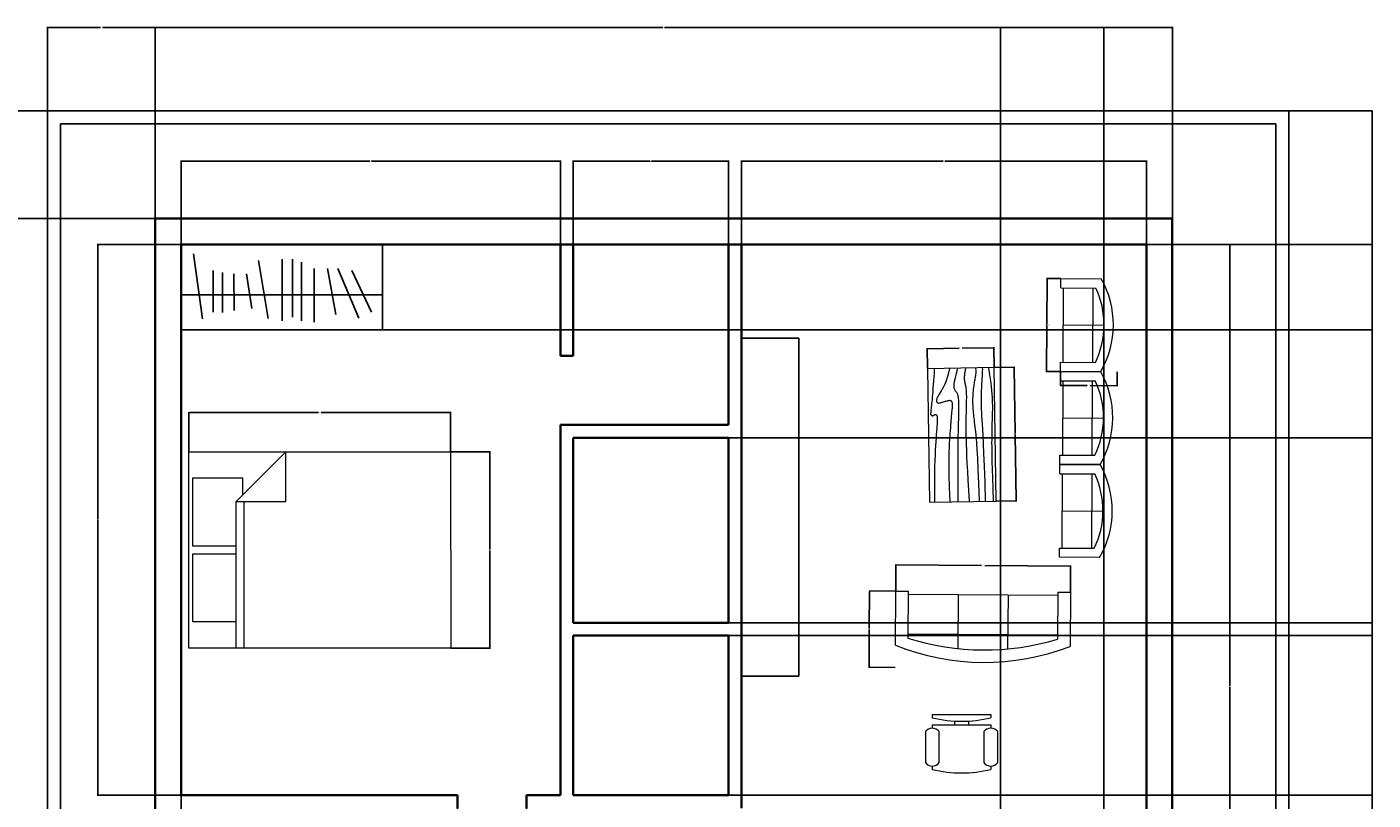
# Model space of a CAD drawing. Units: inches. Extents: x -1085 to 1941, y 1514 to 2348.
# Tile 4 of 9: x -836 to -367, y 2003 to 2272. Entities that reach past the tile are written whole.
import ezdxf

# ---------------------------------------------------------------- set-up
doc = ezdxf.new("R2010")
doc.units = ezdxf.units.IN
for name, color, linetype, lineweight in [('A-ANNO-DIMS', 2, 'Continuous', 18), ('A-FLOR-CASE', 2, 'Continuous', 25), ('A-WALL', 7, 'Continuous', 35), ('C-PROP', 8, 'Continuous', 25), ('FOUNITR-URE', 2, 'Continuous', 18)]:
    doc.layers.add(name, color=color, linetype=linetype, lineweight=lineweight)
doc.styles.get("Standard").update_dxf_attribs({"font": 'arial.ttf'})
doc.dimstyles.get("Standard").update_dxf_attribs({"dimtxt": 0.18, "dimasz": 0.18, "dimexe": 0.18, "dimexo": 0.0625, "dimgap": 0.09, "dimtad": 0, "dimtih": 1, "dimtoh": 1, "dimdec": 4, "dimzin": 0, "dimdsep": 46, "dimtxsty": 'Standard', "dimcen": 0.09, "dimadec": 0, "dimazin": 0, "dimtfac": 1, "dimtdec": 4, "dimtofl": 0, "dimtmove": 0, "dimatfit": 3, "dimfxl": 1, "dimtolj": 1, "dimtzin": 0, "dimarcsym": 0})

# ---------------------------------------------------------------- blocks, each defined once
blk = doc.blocks.new('Bed - Queen')
for p, q in [((0, -80.00003), (0, 0)), ((0, 0), (59.99999, 0)), ((59.99999, 0), (59.99999, -80.00003)), ((7.99999, -1.2), (28.79998, -1.2)), ((7.99999, -14.4), (7.99999, -1.2)), ((28.79998, -1.2), (28.79998, -14.4)), ((31.19999, -1.2), (51.99999, -1.2)), ((31.19999, -14.4), (31.19999, -1.2)), ((51.99999, -1.2), (51.99999, -16.4)), ((0, -14.4), (44.8, -14.4)), ((59.99999, -29.6), (44.8, -14.4)), ((44.8, -14.4), (44.8, -29.6)), ((51.99999, -16.4), (46.79936, -16.4)), ((44.8, -16.8), (0, -16.8)), ((44.8, -29.6), (59.99999, -29.6)), ((59.99999, -80.00003), (0, -80.00003))]:
    blk.add_line(p, q)
blk = doc.blocks.new('Chair - Desk')
for p, q in [((-8.5, 0), (-8.5, -1)), ((-8.5, 0), (8.5, 0)), ((8.5, 0), (8.5, -1)), ((-8.5, -3), (-8.5, -4)), ((-8.5, -3), (8.5, -3)), ((-2, -3), (-2, -1.9355)), ((2, -1.9576), (2, -3)), ((8.5, -3), (8.5, -4)), ((-10.5, -5), (-10.5, -14)), ((-6.5, -14), (-6.5, -5)), ((6.5, -5), (6.5, -14)), ((10.5, -14), (10.5, -5)), ((-8.5, -15), (-8.5, -16)), ((8.5, -15), (8.5, -16))]:
    blk.add_line(p, q)
for centre, radius, start, end in [((0, 34.625), 36.625, 256.5803, 283.4197), ((-8.5, -6.5), 2.5, 36.8699, 143.1301), ((8.5, -6.5), 2.5, 36.8699, 143.1301), ((-8.5, -12.5), 2.5, 216.8699, 323.1301), ((8.5, -12.5), 2.5, 216.8699, 323.1301), ((0, 19.625), 36.625, 256.5803, 283.4197)]:
    blk.add_arc(centre, radius, start, end)
blk = doc.blocks.new('Sofa - Roundback Loveseat 5 ft.')
for p, q in [((0, -32.44198), (0, -5.99998)), ((-24, -33.99998), (-24, -11.46958)), ((-23.9998, -13.38178), (23.99986, -13.38178)), ((24.00004, -33.99998), (24.00004, -11.46958)), ((-24, -32.44198), (24.00004, -32.44198))]:
    blk.add_line(p, q)
for points in [[(-24, -33.99998), (-30, -33.99998), (-30, -7.99998)], [(30.00004, -7.99998), (30.00004, -33.99998), (24.00004, -33.99998)]]:
    blk.add_lwpolyline(points)
for centre, radius, start, end in [((0, -60.24998), 60.24998, 60.13715, 119.8628), ((0, -61.38438), 55.38444, 64.32083, 115.6792)]:
    blk.add_arc(centre, radius, start, end)
blk = doc.blocks.new('Sofa - Roundback 7 ft.')
for p, q in [((-36.000027, -34), (-36.000027, -11.4696)), ((-12.00002, -32.4421), (-12.00003, -6.5971)), ((11.99997, -32.4421), (11.99998, -6.5971)), ((35.99998, -34), (35.99998, -11.4696)), ((-35.999844, -13.3819), (35.9998, -13.3819)), ((-36.000027, -32.4421), (35.99998, -32.4421))]:
    blk.add_line(p, q)
for points in [[(-36.000027, -34), (-42.000027, -34), (-42.000027, -8)], [(41.99998, -8), (41.99998, -34), (35.99998, -34)]]:
    blk.add_lwpolyline(points)
for centre, radius, start, end in [((0, -114.25), 114.25, 68.43141, 111.5686), ((-0.00001, -127.1968), 121.1968, 72.72033, 107.2797)]:
    blk.add_arc(centre, radius, start, end)
blk = doc.blocks.new('Table - Rectangular Woodgrain 60 x 30 in.')
for p, q in [((0, 0), (0, -30)), ((60, 0), (0, 0)), ((60, -30), (60, 0)), ((0, -30), (60, -30))]:
    blk.add_line(p, q)
for points in [[(0, -2.4), (4.8155, -2.418), (9.0302, -2.4688), (12.709, -2.5477), (15.9167, -2.65), (18.7181, -2.7711), (21.1781, -2.9063), (23.3616, -3.0508), (25.3333, -3.2), (27.1477, -3.3495), (28.8172, -3.4958), (30.3437, -3.636), (31.7291, -3.7667), (32.9756, -3.8849), (34.0849, -3.9875), (35.059, -4.0714), (35.9, -4.1334), (36.6114, -4.1711), (37.2041, -4.1854), (37.6906, -4.1779), (38.0833, -4.15), (38.3948, -4.1034), (38.6375, -4.0396), (38.8239, -3.9602), (38.9666, -3.8667), (39.0764, -3.7608), (39.1573, -3.6448), (39.2116, -3.521), (39.2416, -3.3917), (39.2498, -3.2593), (39.2385, -3.1261), (39.21, -2.9944), (39.1666, -2.8667), (39.111, -2.7447), (39.0468, -2.6281), (38.978, -2.5163), (38.9083, -2.4083), (38.8418, -2.3035), (38.7823, -2.201), (38.7337, -2.1001), (38.7, -2), (38.6844, -1.9003), (38.6875, -1.8021), (38.7094, -1.707), (38.75, -1.6167), (38.8094, -1.5326), (38.8875, -1.4563), (38.9844, -1.3893), (39.1, -1.3333), (39.2351, -1.2896), (39.3937, -1.2583), (39.5804, -1.2396), (39.8, -1.2333), (40.057, -1.2396), (40.3562, -1.2583), (40.7023, -1.2896), (41.1, -1.3333), (41.5547, -1.3895), (42.0755, -1.4573), (42.6721, -1.5361), (43.3542, -1.625), (44.1316, -1.7233), (45.014, -1.8302), (46.0114, -1.9449), (47.1333, -2.0667), (48.3862, -2.1947), (49.7625, -2.3281), (51.2513, -2.4663), (52.8416, -2.6083), (54.5226, -2.7535), (56.2833, -2.9011), (58.1127, -3.0501), (60, -3.2)], [(0, -9.2), (6.5759, -9.0858), (11.9385, -9.0365), (16.2527, -9.0418), (19.6833, -9.0917), (22.3952, -9.1759), (24.5531, -9.2844), (26.322, -9.4069), (27.8666, -9.5333), (29.3241, -9.6553), (30.7203, -9.7719), (32.0532, -9.8837), (33.3208, -9.9917), (34.5213, -10.0965), (35.6526, -10.199), (36.7128, -10.2999), (37.7, -10.4), (38.6129, -10.4996), (39.4531, -10.5969), (40.223, -10.6895), (40.925, -10.775), (41.5613, -10.8512), (42.1344, -10.9156), (42.6465, -10.966), (43.1, -11), (43.4976, -11.0158), (43.8437, -11.0136), (44.143, -10.9942), (44.4, -10.9583), (44.6195, -10.9069), (44.8062, -10.8406), (44.9648, -10.7603), (45.1, -10.6667), (45.2155, -10.5598), (45.3114, -10.4365), (45.3871, -10.2929), (45.4416, -10.125), (45.4743, -9.929), (45.4844, -9.7011), (45.4709, -9.4371), (45.4333, -9.1333), (45.3716, -8.7883), (45.2896, -8.4104), (45.1919, -8.0107), (45.0833, -7.6), (44.9685, -7.1893), (44.8521, -6.7896), (44.7388, -6.4117), (44.6333, -6.0667), (44.54, -5.7628), (44.4614, -5.4979), (44.4001, -5.2675), (44.3583, -5.0667), (44.3384, -4.8909), (44.3427, -4.7354), (44.3736, -4.5956), (44.4333, -4.4667), (44.5236, -4.3453), (44.6427, -4.2333), (44.7884, -4.1339), (44.9583, -4.05), (45.1501, -3.9849), (45.3614, -3.9417), (45.59, -3.9234), (45.8333, -3.9333), (46.0915, -3.9749), (46.3734, -4.0531), (46.6906, -4.1736), (47.0542, -4.3417), (47.4756, -4.5629), (47.9661, -4.8427), (48.5372, -5.1866), (49.2, -5.6), (49.9676, -6.0844), (50.8594, -6.625), (51.8965, -7.2031), (53.1, -7.8), (54.491, -8.3969), (56.0906, -8.975), (57.9199, -9.5156), (60, -10)], [(0, -12.8), (5.1847, -12.9322), (9.6213, -13.0323), (13.3963, -13.1059), (16.5958, -13.1583), (19.3063, -13.1952), (21.614, -13.2219), (23.6054, -13.2439), (25.3666, -13.2667), (26.9728, -13.2947), (28.4531, -13.3281), (29.8256, -13.3663), (31.1083, -13.4083), (32.3191, -13.4535), (33.476, -13.501), (34.597, -13.5501), (35.7, -13.6), (36.7984, -13.6497), (37.8875, -13.6979), (38.9578, -13.743), (40, -13.7833), (41.0047, -13.8174), (41.9625, -13.8438), (42.864, -13.8607), (43.7, -13.8667), (44.4631, -13.8604), (45.1552, -13.8417), (45.7801, -13.8104), (46.3416, -13.7667), (46.8439, -13.7104), (47.2906, -13.6417), (47.6858, -13.5604), (48.0333, -13.4667), (48.3375, -13.3608), (48.6042, -13.2448), (48.8396, -13.121), (49.05, -12.9917), (49.2417, -12.8593), (49.4208, -12.7261), (49.5937, -12.5944), (49.7667, -12.4667), (49.9452, -12.3451), (50.1323, -12.2313), (50.3303, -12.1268), (50.5416, -12.0333), (50.7686, -11.9524), (51.0135, -11.8854), (51.2788, -11.8341), (51.5666, -11.8), (51.8785, -11.7843), (52.2116, -11.7865), (52.562, -11.8059), (52.926, -11.8417), (53.2998, -11.8931), (53.6795, -11.9594), (54.0614, -12.0397), (54.4416, -12.1333), (54.8223, -12.2401), (55.2293, -12.3625), (55.6942, -12.5037), (56.2489, -12.6667), (56.9251, -12.8547), (57.7545, -13.0708), (58.7689, -13.3182), (60, -13.6)], [(0, -18), (5.124, -17.7273), (9.6609, -17.5057), (13.6705, -17.3303), (17.2125, -17.1958), (20.3467, -17.0973), (23.1328, -17.0297), (25.6307, -16.9878), (27.9, -16.9667), (29.9928, -16.9617), (31.9302, -16.9703), (33.7254, -16.9907), (35.3917, -17.0208), (36.9423, -17.0588), (38.3906, -17.1026), (39.7499, -17.1503), (41.0333, -17.2), (42.2519, -17.2496), (43.4073, -17.2969), (44.4986, -17.3395), (45.525, -17.375), (46.4858, -17.4012), (47.3802, -17.4156), (48.2074, -17.416), (48.9667, -17.4), (49.6583, -17.3662), (50.2872, -17.3167), (50.8595, -17.2547), (51.3812, -17.1833), (51.8584, -17.1057), (52.2971, -17.025), (52.7034, -16.9443), (53.0833, -16.8667), (53.443, -16.7951), (53.789, -16.7313), (54.128, -16.6768), (54.4666, -16.6334), (54.8115, -16.6024), (55.1693, -16.5854), (55.5465, -16.5841), (55.95, -16.6), (56.3828, -16.6337), (56.8346, -16.6823), (57.2915, -16.7418), (57.7396, -16.8084), (58.165, -16.878), (58.5539, -16.9469), (58.8924, -17.0111), (59.1666, -17.0667), (59.3679, -17.1107), (59.5078, -17.1438), (59.6032, -17.1675), (59.6708, -17.1833), (59.7275, -17.193), (59.7901, -17.1979), (59.8753, -17.1998), (60, -17.2)], [(0, -22.4), (8.0098, -22.2501), (14.4094, -22.1011), (19.4168, -21.9535), (23.25, -21.8083), (26.1269, -21.6663), (28.2656, -21.5281), (29.884, -21.3947), (31.2, -21.2667), (32.3967, -21.1448), (33.5172, -21.0292), (34.5697, -20.9198), (35.5625, -20.8167), (36.5037, -20.7198), (37.4015, -20.6292), (38.2642, -20.5448), (39.1, -20.4667), (39.9164, -20.3951), (40.7187, -20.3313), (41.5117, -20.2768), (42.3, -20.2333), (43.0883, -20.2024), (43.8812, -20.1854), (44.6836, -20.1841), (45.5, -20.2), (46.3328, -20.234), (47.1747, -20.2844), (48.0163, -20.3488), (48.8479, -20.425), (49.66, -20.5106), (50.4429, -20.6031), (51.1872, -20.7004), (51.8833, -20.8), (52.5246, -20.8999), (53.1166, -20.9995), (53.6681, -21.0983), (54.1875, -21.1958), (54.6834, -21.2919), (55.1646, -21.3859), (55.6394, -21.4777), (56.1167, -21.5667), (56.6028, -21.6515), (57.0961, -21.7266), (57.5929, -21.7852), (58.0896, -21.8208), (58.5823, -21.8268), (59.0674, -21.7964), (59.5412, -21.723), (60, -21.6)], [(0, -25.2), (8.6355, -25.0504), (15.7026, -24.9031), (21.4049, -24.7606), (25.9458, -24.625), (29.529, -24.4988), (32.3578, -24.3844), (34.6359, -24.284), (36.5667, -24.2), (38.3213, -24.1341), (39.9417, -24.0854), (41.437, -24.0523), (42.8167, -24.0333), (44.0901, -24.0268), (45.2667, -24.0313), (46.3557, -24.0451), (47.3667, -24.0667), (48.309, -24.0947), (49.1928, -24.1287), (50.0284, -24.168), (50.826, -24.2125), (51.5959, -24.2617), (52.3483, -24.3151), (53.0935, -24.3725), (53.8417, -24.4334), (54.6009, -24.497), (55.3699, -24.561), (56.1454, -24.6226), (56.9239, -24.6792), (57.7021, -24.7279), (58.4764, -24.7662), (59.2435, -24.7911), (60, -24.8)], [(0, -28.8), (5.6867, -28.6681), (10.45, -28.5698), (14.407, -28.5012), (17.675, -28.4584), (20.3711, -28.4374), (22.6125, -28.4344), (24.5164, -28.4455), (26.2, -28.4667), (27.762, -28.4947), (29.2276, -28.5281), (30.6033, -28.5663), (31.8958, -28.6084), (33.1118, -28.6535), (34.2578, -28.7011), (35.3405, -28.7501), (36.3666, -28.8), (37.3443, -28.8497), (38.288, -28.8974), (39.2137, -28.9412), (40.1375, -28.9792), (41.0753, -29.0093), (42.0432, -29.0297), (43.0572, -29.0384), (44.1333, -29.0333), (45.2936, -29.0114), (46.5843, -28.9641), (48.0579, -28.8816), (49.7666, -28.7542), (51.7629, -28.5721), (54.0989, -28.3255), (56.8272, -28.0048), (60, -27.6)]]:
    blk.add_lwpolyline(points)
blk = doc.blocks.new('*D36')
at = {"layer": 'A-ANNO-DIMS', "color": 0, "lineweight": -2, "transparency": 16777216}
for p, q in [((-779.4, 2124.23), (-779.4, 2138.01)), ((-779.22, 2137.83), (-734.35, 2137.84)), ((-688.49, 2137.86), (-733.36, 2137.84)), ((-688.3, 2124.25), (-688.31, 2138.04))]:
    blk.add_line(p, q, dxfattribs=at)
at = {"layer": 'A-ANNO-DIMS', "color": 0, "transparency": 16777216}
for points in [[(-779.22, 2137.86), (-779.22, 2137.8), (-779.4, 2137.83)], [(-688.49, 2137.89), (-688.49, 2137.83), (-688.31, 2137.86)]]:
    blk.add_solid(points, dxfattribs=at)
at = {"layer": 'Defpoints', "color": 0, "transparency": 16777216}
for p in [(-779.4, 2137.83), (-779.4, 2124.17), (-688.3, 2124.19)]:
    blk.add_point(p, dxfattribs=at)
at = {"layer": 'A-ANNO-DIMS', "color": 0, "transparency": 16777216, "insert": (-733.86, 2137.84), "char_height": 0.18, "attachment_point": 5}
blk.add_mtext('\\A1;BED 91', dxfattribs=at)
blk = doc.blocks.new('*D37')
at = {"layer": 'A-ANNO-DIMS', "color": 0, "lineweight": -2, "transparency": 16777216}
for p, q in [((-688.24, 2124.19), (-674.46, 2124.2)), ((-674.64, 2124.02), (-674.63, 2090.22)), ((-674.62, 2056.05), (-674.63, 2089.85)), ((-688.22, 2055.87), (-674.44, 2055.87))]:
    blk.add_line(p, q, dxfattribs=at)
at = {"layer": 'A-ANNO-DIMS', "color": 0, "transparency": 16777216}
for points in [[(-674.61, 2124.02), (-674.67, 2124.02), (-674.64, 2124.2)], [(-674.59, 2056.05), (-674.65, 2056.05), (-674.62, 2055.87)]]:
    blk.add_solid(points, dxfattribs=at)
at = {"layer": 'Defpoints', "color": 0, "transparency": 16777216}
for p in [(-688.3, 2124.19), (-674.64, 2124.2), (-688.28, 2055.87)]:
    blk.add_point(p, dxfattribs=at)
at = {"layer": 'A-ANNO-DIMS', "color": 0, "transparency": 16777216, "insert": (-674.63, 2090.03), "char_height": 0.18, "attachment_point": 5}
blk.add_mtext('\\A1;68', dxfattribs=at)
blk = doc.blocks.new('*D38')
at = {"layer": 'A-ANNO-DIMS', "color": 0, "lineweight": -2, "transparency": 16777216}
for p, q in [((-475.93, 2184.49), (-480.9, 2184.52)), ((-480.72, 2184.34), (-480.81, 2168.53)), ((-480.9, 2152.35), (-480.81, 2168.16)), ((-476.12, 2152.14), (-481.09, 2152.17))]:
    blk.add_line(p, q, dxfattribs=at)
at = {"layer": 'A-ANNO-DIMS', "color": 0, "transparency": 16777216}
for points in [[(-480.75, 2184.34), (-480.69, 2184.34), (-480.72, 2184.52)], [(-480.93, 2152.35), (-480.87, 2152.35), (-480.91, 2152.17)]]:
    blk.add_solid(points, dxfattribs=at)
at = {"layer": 'Defpoints', "color": 0, "transparency": 16777216}
for p in [(-475.87, 2184.49), (-480.91, 2152.17), (-476.05, 2152.14)]:
    blk.add_point(p, dxfattribs=at)
at = {"layer": 'A-ANNO-DIMS', "color": 0, "transparency": 16777216, "insert": (-480.81, 2168.34), "char_height": 0.18, "attachment_point": 5}
blk.add_mtext('\\A1;LOVESEAT 32 TYP.', dxfattribs=at)
blk = doc.blocks.new('*D39')
at = {"layer": 'A-ANNO-DIMS', "color": 0, "lineweight": -2, "transparency": 16777216}
for p, q in [((-476.05, 2152.08), (-476.08, 2147.11)), ((-456.29, 2151.97), (-456.31, 2147)), ((-475.9, 2147.29), (-466.73, 2147.24)), ((-456.49, 2147.18), (-465.67, 2147.23))]:
    blk.add_line(p, q, dxfattribs=at)
at = {"layer": 'A-ANNO-DIMS', "color": 0, "transparency": 16777216}
for points in [[(-475.9, 2147.32), (-475.9, 2147.26), (-476.08, 2147.29)], [(-456.49, 2147.21), (-456.49, 2147.15), (-456.31, 2147.18)]]:
    blk.add_solid(points, dxfattribs=at)
at = {"layer": 'Defpoints', "color": 0, "transparency": 16777216}
for p in [(-476.05, 2152.14), (-456.29, 2152.03), (-456.31, 2147.18)]:
    blk.add_point(p, dxfattribs=at)
at = {"layer": 'A-ANNO-DIMS', "color": 0, "transparency": 16777216, "insert": (-466.2, 2147.23), "char_height": 0.18, "attachment_point": 5}
blk.add_mtext('\\A1;20 TYP.', dxfattribs=at)
blk = doc.blocks.new('*D44')
at = {"layer": 'A-ANNO-DIMS', "color": 0, "lineweight": -2, "transparency": 16777216}
for p, q in [((-533.37, 2075.73), (-533.31, 2084.97)), ((-533.13, 2084.79), (-503.49, 2084.59)), ((-472.7, 2084.39), (-502.34, 2084.59)), ((-472.58, 2075.33), (-472.52, 2084.57))]:
    blk.add_line(p, q, dxfattribs=at)
at = {"layer": 'A-ANNO-DIMS', "color": 0, "transparency": 16777216}
for points in [[(-533.13, 2084.82), (-533.13, 2084.76), (-533.31, 2084.79)], [(-472.7, 2084.42), (-472.7, 2084.36), (-472.52, 2084.39)]]:
    blk.add_solid(points, dxfattribs=at)
at = {"layer": 'Defpoints', "color": 0, "transparency": 16777216}
for p in [(-533.31, 2084.79), (-533.37, 2075.67), (-472.58, 2075.27)]:
    blk.add_point(p, dxfattribs=at)
at = {"layer": 'A-ANNO-DIMS', "color": 0, "transparency": 16777216, "insert": (-502.92, 2084.59), "char_height": 0.18, "attachment_point": 5}
blk.add_mtext('\\A1;SOFA 61', dxfattribs=at)
blk = doc.blocks.new('*D45')
at = {"layer": 'A-ANNO-DIMS', "color": 0, "lineweight": -2, "transparency": 16777216}
for p, q in [((-533.44, 2075.67), (-542.67, 2075.73)), ((-542.5, 2075.55), (-542.58, 2062.64)), ((-542.67, 2049.37), (-542.58, 2062.28)), ((-533.61, 2049.13), (-542.85, 2049.19))]:
    blk.add_line(p, q, dxfattribs=at)
at = {"layer": 'A-ANNO-DIMS', "color": 0, "transparency": 16777216}
for points in [[(-542.53, 2075.55), (-542.47, 2075.55), (-542.49, 2075.73)], [(-542.7, 2049.37), (-542.64, 2049.37), (-542.67, 2049.19)]]:
    blk.add_solid(points, dxfattribs=at)
at = {"layer": 'Defpoints', "color": 0, "transparency": 16777216}
for p in [(-533.37, 2075.67), (-542.67, 2049.19), (-533.55, 2049.13)]:
    blk.add_point(p, dxfattribs=at)
at = {"layer": 'A-ANNO-DIMS', "color": 0, "transparency": 16777216, "insert": (-542.58, 2062.46), "char_height": 0.18, "attachment_point": 5}
blk.add_mtext('\\A1;27', dxfattribs=at)
blk = doc.blocks.new('*D50')
at = {"layer": 'A-ANNO-DIMS', "color": 0, "lineweight": -2, "transparency": 16777216}
for p, q in [((-499.03, 2153.46), (-491.95, 2153.58)), ((-492.13, 2153.39), (-491.77, 2130.54)), ((-491.4, 2107.32), (-491.76, 2130.18)), ((-498.3, 2107.03), (-491.22, 2107.15))]:
    blk.add_line(p, q, dxfattribs=at)
at = {"layer": 'A-ANNO-DIMS', "color": 0, "transparency": 16777216}
for points in [[(-492.1, 2153.39), (-492.16, 2153.39), (-492.13, 2153.57)], [(-491.37, 2107.32), (-491.43, 2107.32), (-491.4, 2107.14)]]:
    blk.add_solid(points, dxfattribs=at)
at = {"layer": 'Defpoints', "color": 0, "transparency": 16777216}
for p in [(-499.1, 2153.46), (-492.13, 2153.57), (-498.36, 2107.03)]:
    blk.add_point(p, dxfattribs=at)
at = {"layer": 'A-ANNO-DIMS', "color": 0, "transparency": 16777216, "insert": (-491.77, 2130.36), "char_height": 0.18, "attachment_point": 5}
blk.add_mtext('\\A1;TABLE 46 TYP.', dxfattribs=at)
blk = doc.blocks.new('*D51')
at = {"layer": 'A-ANNO-DIMS', "color": 0, "lineweight": -2, "transparency": 16777216}
for p, q in [((-522.31, 2153.16), (-522.42, 2160.24)), ((-522.24, 2160.06), (-511.34, 2160.24)), ((-499.39, 2160.42), (-510.28, 2160.25)), ((-499.1, 2153.53), (-499.21, 2160.61))]:
    blk.add_line(p, q, dxfattribs=at)
at = {"layer": 'A-ANNO-DIMS', "color": 0, "transparency": 16777216}
for points in [[(-522.24, 2160.09), (-522.24, 2160.03), (-522.42, 2160.06)], [(-499.39, 2160.45), (-499.39, 2160.39), (-499.21, 2160.43)]]:
    blk.add_solid(points, dxfattribs=at)
at = {"layer": 'Defpoints', "color": 0, "transparency": 16777216}
for p in [(-522.42, 2160.06), (-522.31, 2153.1), (-499.1, 2153.46)]:
    blk.add_point(p, dxfattribs=at)
at = {"layer": 'A-ANNO-DIMS', "color": 0, "transparency": 16777216, "insert": (-510.81, 2160.24), "char_height": 0.18, "attachment_point": 5}
blk.add_mtext('\\A1;23 TYP.', dxfattribs=at)
blk = doc.blocks.new('*D95')
at = {"layer": 'A-ANNO-DIMS', "color": 0, "lineweight": -2, "transparency": 16777216}
for p, q in [((-396.54, 2242.88), (-367.42, 2242.88)), ((-367.6, 2242.7), (-367.6, 1955.07)), ((-367.6, 1667.06), (-367.6, 1954.7)), ((-396.54, 1666.88), (-367.42, 1666.88))]:
    blk.add_line(p, q, dxfattribs=at)
at = {"layer": 'A-ANNO-DIMS', "color": 0, "transparency": 16777216}
for points in [[(-367.63, 2242.7), (-367.57, 2242.7), (-367.6, 2242.88)], [(-367.63, 1667.06), (-367.57, 1667.06), (-367.6, 1666.88)]]:
    blk.add_solid(points, dxfattribs=at)
at = {"layer": 'Defpoints', "color": 0, "transparency": 16777216}
for p in [(-396.6, 2242.88), (-367.6, 2242.88), (-396.6, 1666.88)]:
    blk.add_point(p, dxfattribs=at)
at = {"layer": 'A-ANNO-DIMS', "color": 0, "transparency": 16777216, "insert": (-367.6, 1954.88), "char_height": 0.18, "attachment_point": 5}
blk.add_mtext('\\A1;576', dxfattribs=at)
blk = doc.blocks.new('*D96')
at = {"layer": 'A-ANNO-DIMS', "color": 0, "lineweight": -2, "transparency": 16777216}
for p, q in [((-791.1, 2205.45), (-791.1, 2272.06)), ((-790.92, 2271.88), (-614.39, 2271.88)), ((-437.28, 2271.88), (-613.81, 2271.88)), ((-437.1, 2205.45), (-437.1, 2272.06))]:
    blk.add_line(p, q, dxfattribs=at)
at = {"layer": 'A-ANNO-DIMS', "color": 0, "transparency": 16777216}
for points in [[(-790.92, 2271.91), (-790.92, 2271.85), (-791.1, 2271.88)], [(-437.28, 2271.91), (-437.28, 2271.85), (-437.1, 2271.88)]]:
    blk.add_solid(points, dxfattribs=at)
at = {"layer": 'Defpoints', "color": 0, "transparency": 16777216}
for p in [(-437.1, 2271.88), (-791.1, 2205.38), (-437.1, 2205.38)]:
    blk.add_point(p, dxfattribs=at)
at = {"layer": 'A-ANNO-DIMS', "color": 0, "transparency": 16777216, "insert": (-614.1, 2271.88), "char_height": 0.18, "attachment_point": 5}
blk.add_mtext('\\A1;354', dxfattribs=at)
blk = doc.blocks.new('*D97')
at = {"layer": 'A-ANNO-DIMS', "color": 0, "lineweight": -2, "transparency": 16777216}
for p, q in [((-791.17, 2205.38), (-857.78, 2205.38)), ((-857.6, 2205.2), (-857.6, 1965.57)), ((-857.6, 1725.56), (-857.6, 1965.2)), ((-791.17, 1725.38), (-857.78, 1725.38))]:
    blk.add_line(p, q, dxfattribs=at)
at = {"layer": 'A-ANNO-DIMS', "color": 0, "transparency": 16777216}
for points in [[(-857.63, 2205.2), (-857.57, 2205.2), (-857.6, 2205.38)], [(-857.63, 1725.56), (-857.57, 1725.56), (-857.6, 1725.38)]]:
    blk.add_solid(points, dxfattribs=at)
at = {"layer": 'Defpoints', "color": 0, "transparency": 16777216}
for p in [(-791.1, 2205.38), (-857.6, 1725.38), (-791.1, 1725.38)]:
    blk.add_point(p, dxfattribs=at)
at = {"layer": 'A-ANNO-DIMS', "color": 0, "transparency": 16777216, "insert": (-857.6, 1965.38), "char_height": 0.18, "attachment_point": 5}
blk.add_mtext('\\A1;480', dxfattribs=at)
blk = doc.blocks.new('*D98')
at = {"layer": 'A-ANNO-DIMS', "color": 0, "lineweight": -2, "transparency": 16777216}
for p, q in [((-828.6, 2242.95), (-828.6, 2272.06)), ((-828.42, 2271.88), (-810.18, 2271.88)), ((-791.28, 2271.88), (-809.53, 2271.88)), ((-791.1, 2205.45), (-791.1, 2272.06))]:
    blk.add_line(p, q, dxfattribs=at)
at = {"layer": 'A-ANNO-DIMS', "color": 0, "transparency": 16777216}
for points in [[(-828.42, 2271.91), (-828.42, 2271.85), (-828.6, 2271.88)], [(-791.28, 2271.91), (-791.28, 2271.85), (-791.1, 2271.88)]]:
    blk.add_solid(points, dxfattribs=at)
at = {"layer": 'Defpoints', "color": 0, "transparency": 16777216}
for p in [(-791.1, 2271.88), (-828.6, 2242.88), (-791.1, 2205.38)]:
    blk.add_point(p, dxfattribs=at)
at = {"layer": 'A-ANNO-DIMS', "color": 0, "transparency": 16777216, "insert": (-809.85, 2271.88), "char_height": 0.18, "attachment_point": 5}
blk.add_mtext('\\A1;37.5', dxfattribs=at)
blk = doc.blocks.new('*D99')
at = {"layer": 'A-ANNO-DIMS', "color": 0, "lineweight": -2, "transparency": 16777216}
for p, q in [((-828.67, 2242.88), (-857.78, 2242.88)), ((-857.6, 2242.7), (-857.6, 2224.32)), ((-857.6, 2205.56), (-857.6, 2223.95)), ((-791.17, 2205.38), (-857.78, 2205.38))]:
    blk.add_line(p, q, dxfattribs=at)
at = {"layer": 'A-ANNO-DIMS', "color": 0, "transparency": 16777216}
for points in [[(-857.63, 2242.7), (-857.57, 2242.7), (-857.6, 2242.88)], [(-857.63, 2205.56), (-857.57, 2205.56), (-857.6, 2205.38)]]:
    blk.add_solid(points, dxfattribs=at)
at = {"layer": 'Defpoints', "color": 0, "transparency": 16777216}
for p in [(-828.6, 2242.88), (-857.6, 2205.38), (-791.1, 2205.38)]:
    blk.add_point(p, dxfattribs=at)
at = {"layer": 'A-ANNO-DIMS', "color": 0, "transparency": 16777216, "insert": (-857.6, 2224.13), "char_height": 0.18, "attachment_point": 5}
blk.add_mtext('\\A1;37.5', dxfattribs=at)
blk = doc.blocks.new('*D100')
at = {"layer": 'A-ANNO-DIMS', "color": 0, "lineweight": -2, "transparency": 16777216}
for p, q in [((-782.1, 2196.45), (-782.1, 2225.56)), ((-781.92, 2225.38), (-716.38, 2225.38)), ((-650.28, 2225.38), (-715.82, 2225.38)), ((-650.1, 2196.45), (-650.1, 2225.56))]:
    blk.add_line(p, q, dxfattribs=at)
at = {"layer": 'A-ANNO-DIMS', "color": 0, "transparency": 16777216}
for points in [[(-781.92, 2225.41), (-781.92, 2225.35), (-782.1, 2225.38)], [(-650.28, 2225.41), (-650.28, 2225.35), (-650.1, 2225.38)]]:
    blk.add_solid(points, dxfattribs=at)
at = {"layer": 'Defpoints', "color": 0, "transparency": 16777216}
for p in [(-650.1, 2225.38), (-782.1, 2196.38), (-650.1, 2196.38)]:
    blk.add_point(p, dxfattribs=at)
at = {"layer": 'A-ANNO-DIMS', "color": 0, "transparency": 16777216, "insert": (-716.1, 2225.38), "char_height": 0.18, "attachment_point": 5}
blk.add_mtext('\\A1;132', dxfattribs=at)
blk = doc.blocks.new('*D101')
at = {"layer": 'A-ANNO-DIMS', "color": 0, "lineweight": -2, "transparency": 16777216}
for p, q in [((-782.17, 2196.38), (-811.28, 2196.38)), ((-811.1, 2196.2), (-811.1, 2100.71)), ((-811.1, 2004.86), (-811.1, 2100.35)), ((-782.17, 2004.68), (-811.28, 2004.68))]:
    blk.add_line(p, q, dxfattribs=at)
at = {"layer": 'A-ANNO-DIMS', "color": 0, "transparency": 16777216}
for points in [[(-811.13, 2196.2), (-811.07, 2196.2), (-811.1, 2196.38)], [(-811.13, 2004.86), (-811.07, 2004.86), (-811.1, 2004.68)]]:
    blk.add_solid(points, dxfattribs=at)
at = {"layer": 'Defpoints', "color": 0, "transparency": 16777216}
for p in [(-811.1, 2196.38), (-782.1, 2196.38), (-782.1, 2004.68)]:
    blk.add_point(p, dxfattribs=at)
at = {"layer": 'A-ANNO-DIMS', "color": 0, "transparency": 16777216, "insert": (-811.1, 2100.53), "char_height": 0.18, "attachment_point": 5}
blk.add_mtext('\\A1;191.7', dxfattribs=at)
blk = doc.blocks.new('*D102')
at = {"layer": 'A-ANNO-DIMS', "color": 0, "lineweight": -2, "transparency": 16777216}
for p, q in [((-645.6, 2196.45), (-645.6, 2225.56)), ((-645.42, 2225.38), (-618.82, 2225.38)), ((-591.78, 2225.38), (-618.38, 2225.38)), ((-591.6, 2196.45), (-591.6, 2225.56))]:
    blk.add_line(p, q, dxfattribs=at)
at = {"layer": 'A-ANNO-DIMS', "color": 0, "transparency": 16777216}
for points in [[(-645.42, 2225.41), (-645.42, 2225.35), (-645.6, 2225.38)], [(-591.78, 2225.41), (-591.78, 2225.35), (-591.6, 2225.38)]]:
    blk.add_solid(points, dxfattribs=at)
at = {"layer": 'Defpoints', "color": 0, "transparency": 16777216}
for p in [(-591.6, 2225.38), (-645.6, 2196.38), (-591.6, 2196.38)]:
    blk.add_point(p, dxfattribs=at)
at = {"layer": 'A-ANNO-DIMS', "color": 0, "transparency": 16777216, "insert": (-618.6, 2225.38), "char_height": 0.18, "attachment_point": 5}
blk.add_mtext('\\A1;54', dxfattribs=at)
blk = doc.blocks.new('*D103')
at = {"layer": 'A-ANNO-DIMS', "color": 0, "lineweight": -2, "transparency": 16777216}
for p, q in [((-645.54, 2060.18), (-367.42, 2060.18)), ((-367.6, 2060), (-367.6, 2032.61)), ((-367.6, 2004.86), (-367.6, 2032.25)), ((-645.54, 2004.68), (-367.42, 2004.68))]:
    blk.add_line(p, q, dxfattribs=at)
at = {"layer": 'A-ANNO-DIMS', "color": 0, "transparency": 16777216}
for points in [[(-367.63, 2060), (-367.57, 2060), (-367.6, 2060.18)], [(-367.63, 2004.86), (-367.57, 2004.86), (-367.6, 2004.68)]]:
    blk.add_solid(points, dxfattribs=at)
at = {"layer": 'Defpoints', "color": 0, "transparency": 16777216}
for p in [(-645.6, 2060.18), (-367.6, 2060.18), (-645.6, 2004.68)]:
    blk.add_point(p, dxfattribs=at)
at = {"layer": 'A-ANNO-DIMS', "color": 0, "transparency": 16777216, "insert": (-367.6, 2032.43), "char_height": 0.18, "attachment_point": 5}
blk.add_mtext('\\A1;55.5', dxfattribs=at)
blk = doc.blocks.new('*D104')
at = {"layer": 'A-ANNO-DIMS', "color": 0, "lineweight": -2, "transparency": 16777216}
for p, q in [((-645.54, 2129.05), (-367.42, 2129.05)), ((-367.6, 2128.87), (-367.6, 2097.05)), ((-367.6, 2064.86), (-367.6, 2096.68)), ((-645.54, 2064.68), (-367.42, 2064.68))]:
    blk.add_line(p, q, dxfattribs=at)
at = {"layer": 'A-ANNO-DIMS', "color": 0, "transparency": 16777216}
for points in [[(-367.63, 2128.87), (-367.57, 2128.87), (-367.6, 2129.05)], [(-367.63, 2064.86), (-367.57, 2064.86), (-367.6, 2064.68)]]:
    blk.add_solid(points, dxfattribs=at)
at = {"layer": 'Defpoints', "color": 0, "transparency": 16777216}
for p in [(-645.6, 2129.05), (-367.6, 2129.05), (-645.6, 2064.68)]:
    blk.add_point(p, dxfattribs=at)
at = {"layer": 'A-ANNO-DIMS', "color": 0, "transparency": 16777216, "insert": (-367.6, 2096.87), "char_height": 0.18, "attachment_point": 5}
blk.add_mtext('\\A1;64.38', dxfattribs=at)
blk = doc.blocks.new('*D105')
at = {"layer": 'A-ANNO-DIMS', "color": 0, "lineweight": -2, "transparency": 16777216}
for p, q in [((-782.04, 2196.38), (-367.42, 2196.38)), ((-367.6, 2196.2), (-367.6, 2181.71)), ((-367.6, 2166.86), (-367.6, 2181.35)), ((-782.04, 2166.68), (-367.42, 2166.68))]:
    blk.add_line(p, q, dxfattribs=at)
at = {"layer": 'A-ANNO-DIMS', "color": 0, "transparency": 16777216}
for points in [[(-367.63, 2196.2), (-367.57, 2196.2), (-367.6, 2196.38)], [(-367.63, 2166.86), (-367.57, 2166.86), (-367.6, 2166.68)]]:
    blk.add_solid(points, dxfattribs=at)
at = {"layer": 'Defpoints', "color": 0, "transparency": 16777216}
for p in [(-782.1, 2196.38), (-782.1, 2166.68), (-367.6, 2166.68)]:
    blk.add_point(p, dxfattribs=at)
at = {"layer": 'A-ANNO-DIMS', "color": 0, "transparency": 16777216, "insert": (-367.6, 2181.53), "char_height": 0.18, "attachment_point": 5}
blk.add_mtext('\\A1;29.706', dxfattribs=at)
blk = doc.blocks.new('*D106')
at = {"layer": 'A-ANNO-DIMS', "color": 0, "lineweight": -2, "transparency": 16777216}
for p, q in [((-685.88, 2004.62), (-685.88, 1637.7)), ((-661.88, 2004.62), (-661.88, 1637.7)), ((-685.7, 1637.88), (-674.1, 1637.88)), ((-662.06, 1637.88), (-673.66, 1637.88))]:
    blk.add_line(p, q, dxfattribs=at)
at = {"layer": 'A-ANNO-DIMS', "color": 0, "transparency": 16777216}
for points in [[(-685.7, 1637.91), (-685.7, 1637.85), (-685.88, 1637.88)], [(-662.06, 1637.91), (-662.06, 1637.85), (-661.88, 1637.88)]]:
    blk.add_solid(points, dxfattribs=at)
at = {"layer": 'Defpoints', "color": 0, "transparency": 16777216}
for p in [(-685.88, 2004.68), (-661.88, 2004.68), (-685.88, 1637.88)]:
    blk.add_point(p, dxfattribs=at)
at = {"layer": 'A-ANNO-DIMS', "color": 0, "transparency": 16777216, "insert": (-673.88, 1637.88), "char_height": 0.18, "attachment_point": 5}
blk.add_mtext('\\A1;24', dxfattribs=at)
blk = doc.blocks.new('*D107')
at = {"layer": 'A-ANNO-DIMS', "color": 0, "lineweight": -2, "transparency": 16777216}
for p, q in [((-782.1, 2004.62), (-782.1, 1637.7)), ((-685.88, 2004.62), (-685.88, 1637.7)), ((-781.92, 1637.88), (-734.38, 1637.88)), ((-686.06, 1637.88), (-733.6, 1637.88))]:
    blk.add_line(p, q, dxfattribs=at)
at = {"layer": 'A-ANNO-DIMS', "color": 0, "transparency": 16777216}
for points in [[(-781.92, 1637.91), (-781.92, 1637.85), (-782.1, 1637.88)], [(-686.06, 1637.91), (-686.06, 1637.85), (-685.88, 1637.88)]]:
    blk.add_solid(points, dxfattribs=at)
at = {"layer": 'Defpoints', "color": 0, "transparency": 16777216}
for p in [(-782.1, 2004.68), (-685.88, 2004.68), (-782.1, 1637.88)]:
    blk.add_point(p, dxfattribs=at)
at = {"layer": 'A-ANNO-DIMS', "color": 0, "transparency": 16777216, "insert": (-733.99, 1637.88), "char_height": 0.18, "attachment_point": 5}
blk.add_mtext('\\A1;96.23', dxfattribs=at)
blk = doc.blocks.new('*D108')
at = {"layer": 'A-ANNO-DIMS', "color": 0, "lineweight": -2, "transparency": 16777216}
for p, q in [((-496.94, 1888.45), (-496.94, 2272.06)), ((-496.76, 2271.88), (-479.16, 2271.88)), ((-461.12, 2271.88), (-478.72, 2271.88)), ((-460.94, 1888.45), (-460.94, 2272.06))]:
    blk.add_line(p, q, dxfattribs=at)
at = {"layer": 'A-ANNO-DIMS', "color": 0, "transparency": 16777216}
for points in [[(-496.76, 2271.91), (-496.76, 2271.85), (-496.94, 2271.88)], [(-461.12, 2271.91), (-461.12, 2271.85), (-460.94, 2271.88)]]:
    blk.add_solid(points, dxfattribs=at)
at = {"layer": 'Defpoints', "color": 0, "transparency": 16777216}
for p in [(-460.94, 2271.88), (-496.94, 1888.38), (-460.94, 1888.38)]:
    blk.add_point(p, dxfattribs=at)
at = {"layer": 'A-ANNO-DIMS', "color": 0, "transparency": 16777216, "insert": (-478.94, 2271.88), "char_height": 0.18, "attachment_point": 5}
blk.add_mtext('\\A1;36', dxfattribs=at)
blk = doc.blocks.new('*D109')
at = {"layer": 'A-ANNO-DIMS', "color": 0, "lineweight": -2, "transparency": 16777216}
for p, q in [((-587.1, 2196.45), (-587.1, 2225.56)), ((-586.92, 2225.38), (-516.87, 2225.38)), ((-446.28, 2225.38), (-516.34, 2225.38)), ((-446.1, 2196.45), (-446.1, 2225.56))]:
    blk.add_line(p, q, dxfattribs=at)
at = {"layer": 'A-ANNO-DIMS', "color": 0, "transparency": 16777216}
for points in [[(-586.92, 2225.41), (-586.92, 2225.35), (-587.1, 2225.38)], [(-446.28, 2225.41), (-446.28, 2225.35), (-446.1, 2225.38)]]:
    blk.add_solid(points, dxfattribs=at)
at = {"layer": 'Defpoints', "color": 0, "transparency": 16777216}
for p in [(-446.1, 2225.38), (-587.1, 2196.38), (-446.1, 2196.38)]:
    blk.add_point(p, dxfattribs=at)
at = {"layer": 'A-ANNO-DIMS', "color": 0, "transparency": 16777216, "insert": (-516.6, 2225.38), "char_height": 0.18, "attachment_point": 5}
blk.add_mtext('\\A1;141', dxfattribs=at)
blk = doc.blocks.new('*D110')
at = {"layer": 'A-ANNO-DIMS', "color": 0, "lineweight": -2, "transparency": 16777216}
for p, q in [((-446.04, 2196.38), (-416.92, 2196.38)), ((-417.1, 2196.2), (-417.1, 2042.57)), ((-417.1, 1888.56), (-417.1, 2042.2)), ((-446.04, 1888.38), (-416.92, 1888.38))]:
    blk.add_line(p, q, dxfattribs=at)
at = {"layer": 'A-ANNO-DIMS', "color": 0, "transparency": 16777216}
for points in [[(-417.13, 2196.2), (-417.07, 2196.2), (-417.1, 2196.38)], [(-417.13, 1888.56), (-417.07, 1888.56), (-417.1, 1888.38)]]:
    blk.add_solid(points, dxfattribs=at)
at = {"layer": 'Defpoints', "color": 0, "transparency": 16777216}
for p in [(-446.1, 2196.38), (-446.1, 1888.38), (-417.1, 1888.38)]:
    blk.add_point(p, dxfattribs=at)
at = {"layer": 'A-ANNO-DIMS', "color": 0, "transparency": 16777216, "insert": (-417.1, 2042.38), "char_height": 0.18, "attachment_point": 5}
blk.add_mtext('\\A1;308', dxfattribs=at)

msp = doc.modelspace()

# ---------------------------------------------------------------- linework, layer by layer
at = {"layer": 'A-FLOR-CASE'}
for p, q in [((-777.8027, 2193.1085), (-774.6755, 2170.4108)), ((-712.0452, 2196.3835), (-712.0452, 2166.6777)), ((-755.2197, 2190.7548), (-751.8524, 2170.5633)), ((-746.9712, 2191.1675), (-746.9712, 2169.8172)), ((-743.3297, 2191.1675), (-743.3297, 2171.0303)), ((-740.1737, 2190.197), (-740.1737, 2169.8172)), ((-771.0052, 2187.2856), (-771.0052, 2172.7286)), ((-767.7218, 2186.6024), (-767.7218, 2172.6322)), ((-763.7279, 2186.1272), (-763.6328, 2173.3925)), ((-759.3432, 2186.16), (-757.5156, 2174.0815)), ((-735.8039, 2188.0135), (-735.8039, 2169.3187)), ((-731.1914, 2188.0135), (-728.2684, 2171.9583)), ((-727.5498, 2188.0135), (-720.2154, 2170.7121)), ((-722.6945, 2187.2856), (-715.897, 2172.7286)), ((-782.1032, 2178.794), (-712.0452, 2178.794)), ((-782.1032, 2166.6777), (-650.1032, 2166.6777)), ((-567.0781, 2163.7686), (-587.1032, 2163.7686)), ((-567.0781, 2046.0746), (-567.0781, 2163.7686)), ((-587.1032, 2046.0746), (-567.0781, 2046.0746))]:
    msp.add_line(p, q, dxfattribs=at)
at = {"layer": 'A-WALL'}
for p, q in [((-791.1032, 2205.3835), (-437.1032, 2205.3835)), ((-791.1032, 1888.3835), (-791.1032, 2205.3835)), ((-437.1032, 2205.3835), (-437.1032, 1888.7098)), ((-782.1032, 2196.3835), (-446.1032, 2196.3835)), ((-782.1032, 2004.6777), (-782.1032, 2196.3835)), ((-650.1032, 2166.6777), (-650.1032, 2196.3835)), ((-650.1032, 2196.3835), (-650.1032, 2166.6777)), ((-645.6032, 2196.3835), (-645.6032, 2166.6777)), ((-591.6032, 2191.731), (-591.6032, 2196.3835)), ((-587.1032, 2191.731), (-587.1032, 2196.3835)), ((-446.1032, 2196.3835), (-446.1032, 1888.3835)), ((-591.6032, 2133.554), (-591.6032, 2191.731)), ((-587.1032, 2129.054), (-587.1032, 2191.731)), ((-650.1032, 2166.6777), (-650.1032, 2157.554)), ((-645.6032, 2166.6777), (-645.6032, 2157.554)), ((-650.1032, 2157.554), (-645.6032, 2157.554)), ((-645.6032, 2133.554), (-650.1032, 2133.554)), ((-650.1032, 2133.554), (-650.1032, 2004.6777)), ((-645.6032, 2133.554), (-591.6032, 2133.554)), ((-645.6032, 2129.054), (-645.6032, 2064.6777)), ((-645.6032, 2129.054), (-591.6032, 2129.054)), ((-591.6032, 2064.6777), (-591.6032, 2129.054)), ((-587.1032, 2000.1777), (-587.1032, 2129.054)), ((-645.6032, 2064.6777), (-591.6032, 2064.6777)), ((-645.6032, 2060.1777), (-591.6032, 2060.1777)), ((-645.6032, 2060.1777), (-645.6032, 2004.6777)), ((-591.6032, 2060.1777), (-591.6032, 2004.6777)), ((-685.8764, 2004.6777), (-782.1032, 2004.6777)), ((-685.8764, 2000.1777), (-685.8764, 2004.6777)), ((-650.1032, 2004.6777), (-661.8764, 2004.6777)), ((-661.8764, 2004.6777), (-661.8764, 2000.1777)), ((-645.6032, 2004.6777), (-591.6032, 2004.6777))]:
    msp.add_line(p, q, dxfattribs=at)
at = {"layer": 'C-PROP'}
for p, q in [((-828.6032, 2242.8835), (-396.6032, 2242.8835)), ((-828.6032, 1666.8835), (-828.6032, 2242.8835)), ((-396.6032, 2242.8835), (-396.6032, 1666.8835)), ((-824.1032, 2238.3835), (-401.1032, 2238.3835)), ((-824.1032, 1671.3835), (-824.1032, 2238.3835)), ((-401.1032, 2238.3835), (-401.1032, 1671.3835))]:
    msp.add_line(p, q, dxfattribs=at)

# ---------------------------------------------------------------- block references
at = {"layer": 'FOUNITR-URE'}
for name, p, xscale, yscale, zscale, rotation in [('Sofa - Roundback Loveseat 5 ft.', (-457.6294, 2168.2104), 0.5391437841071741, 0.5391437841071741, 0.5391437841071741, 269.6684342890045), ('Table - Rectangular Woodgrain 60 x 30 in.', (-521.5789, 2106.6662), 0.7739415990810241, 0.7739415990810241, 0.7739415990810241, 90.90402502805208), ('Sofa - Roundback Loveseat 5 ft.', (-457.8166, 2135.8623), 0.5391437841071741, 0.5391437841071741, 0.5391437841071741, 269.6684342890045), ('Bed - Queen', (-779.3818, 2055.8432), 1.138726013966516, 1.138726013966516, 1.138726013966516, 90.01605390430686), ('Sofa - Roundback Loveseat 5 ft.', (-458.0038, 2103.5142), 0.5391437841071741, 0.5391437841071741, 0.5391437841071741, 269.6684342890045), ('Sofa - Roundback 7 ft.', (-503.1381, 2050.8632), 0.7237795177670652, 0.7237795177670652, 0.7237795177670652, 179.6235229613476)]:
    msp.add_blockref(name, p, dxfattribs=dict(at, xscale=xscale, yscale=yscale, zscale=zscale, rotation=rotation))
at = {"layer": 'FOUNITR-URE', "xscale": 1.198560681527003, "yscale": 1.198560681527003, "zscale": 1.198560681527003}
msp.add_blockref('Chair - Desk', (-510.4657, 2032.7864), dxfattribs=at)

# ---------------------------------------------------------------- dimensions: what is measured, and where the dimension line sits
at = {"layer": 'A-ANNO-DIMS'}
for base, p1, p2, override, picture, middle in [((-791.1032, 2271.8835), (-828.6032, 2242.8835), (-791.1032, 2205.3835), {"dimdec": 1, "dimlfac": 1, "dimrnd": 0, "dimzin": 0, "dimdsep": 46, "dimlunit": 2}, '*D98', (-809.8532, 2271.8835)), ((-437.1032, 2271.8835), (-791.1032, 2205.3835), (-437.1032, 2205.3835), {"dimdec": 0, "dimlfac": 1, "dimrnd": 0, "dimzin": 0, "dimdsep": 46, "dimlunit": 2}, '*D96', (-614.1032, 2271.8835)), ((-460.941, 2271.8835), (-496.941, 1888.3835), (-460.941, 1888.3835), {"dimdec": 0, "dimlfac": 1, "dimrnd": 0, "dimzin": 0, "dimdsep": 46, "dimlunit": 2}, '*D108', (-478.941, 2271.8835)), ((-650.1032, 2225.3835), (-782.1032, 2196.3835), (-650.1032, 2196.3835), {"dimdec": 0, "dimlfac": 1, "dimrnd": 0, "dimzin": 0, "dimdsep": 46, "dimlunit": 2}, '*D100', (-716.1032, 2225.3835)), ((-591.6032, 2225.3835), (-645.6032, 2196.3835), (-591.6032, 2196.3835), {"dimdec": 0, "dimlfac": 1, "dimrnd": 0, "dimzin": 0, "dimdsep": 46, "dimlunit": 2}, '*D102', (-618.6032, 2225.3835)), ((-446.1032, 2225.3835), (-587.1032, 2196.3835), (-446.1032, 2196.3835), {"dimdec": 0, "dimlfac": 1, "dimrnd": 0, "dimzin": 0, "dimdsep": 46, "dimlunit": 2}, '*D109', (-516.6032, 2225.3835)), ((-782.1032, 1637.8835), (-685.8764, 2004.6777), (-782.1032, 2004.6777), {"dimdec": 2, "dimlfac": 1, "dimrnd": 0, "dimzin": 0, "dimdsep": 46, "dimlunit": 2}, '*D107', (-733.9898, 1637.8835)), ((-685.8764, 1637.8835), (-661.8764, 2004.6777), (-685.8764, 2004.6777), {"dimdec": 0, "dimlfac": 1, "dimrnd": 0, "dimzin": 0, "dimdsep": 46, "dimlunit": 2}, '*D106', (-673.8764, 1637.8835))]:
    dim = msp.add_linear_dim(base=base, p1=p1, p2=p2, dimstyle='Standard', override=override, dxfattribs=at)
    dim.commit()
    dim.dimension.update_dxf_attribs({"geometry": picture, "text_midpoint": middle})
for base, p1, p2, angle, override, picture, middle in [((-857.6032, 2205.3835), (-828.6032, 2242.8835), (-791.1032, 2205.3835), 90, {"dimdec": 1, "dimlfac": 1, "dimrnd": 0, "dimzin": 0, "dimdsep": 46, "dimlunit": 2}, '*D99', (-857.6032, 2224.1335)), ((-367.6032, 2242.8835), (-396.6032, 1666.8835), (-396.6032, 2242.8835), 90, {"dimdec": 0, "dimlfac": 1, "dimrnd": 0, "dimzin": 0, "dimdsep": 46, "dimlunit": 2}, '*D95', (-367.6032, 1954.8835)), ((-857.6032, 1725.3835), (-791.1032, 2205.3835), (-791.1032, 1725.3835), 90, {"dimdec": 0, "dimlfac": 1, "dimrnd": 0, "dimzin": 0, "dimdsep": 46, "dimlunit": 2}, '*D97', (-857.6032, 1965.3835)), ((-811.1032, 2196.3835), (-782.1032, 2004.6777), (-782.1032, 2196.3835), 90, {"dimdec": 1, "dimlfac": 1, "dimrnd": 0, "dimzin": 0, "dimdsep": 46, "dimlunit": 2}, '*D101', (-811.1032, 2100.5306)), ((-367.6032, 2166.6777), (-782.1032, 2196.3835), (-782.1032, 2166.6777), 90, {"dimdec": 3, "dimlfac": 1, "dimrnd": 0, "dimzin": 0, "dimdsep": 46, "dimlunit": 2}, '*D105', (-367.6032, 2181.5306)), ((-417.1032, 1888.3835), (-446.1032, 2196.3835), (-446.1032, 1888.3835), 270, {"dimdec": 0, "dimlfac": 1, "dimrnd": 0, "dimzin": 0, "dimdsep": 46, "dimlunit": 2}, '*D110', (-417.1032, 2042.3835)), ((-367.6032, 2129.054), (-645.6032, 2064.6777), (-645.6032, 2129.054), 90, {"dimdec": 2, "dimlfac": 1, "dimrnd": 0, "dimzin": 0, "dimdsep": 46, "dimlunit": 2}, '*D104', (-367.6032, 2096.8659)), ((-674.6381, 2124.1961), (-688.2837, 2055.8687), (-688.3028, 2124.1923), 90.016054, {"dimdec": 0, "dimlfac": 1, "dimrnd": 0, "dimzin": 0, "dimdsep": 46, "dimlunit": 2}, '*D37', (-674.6285, 2090.0344)), ((-542.6683, 2049.1929), (-533.3745, 2075.671), (-533.5488, 2049.1329), 269.623523, {"dimdec": 0, "dimlfac": 1, "dimrnd": 0, "dimzin": 0, "dimdsep": 46, "dimlunit": 2}, '*D45', (-542.5811, 2062.4619)), ((-367.6032, 2060.1777), (-645.6032, 2004.6777), (-645.6032, 2060.1777), 90, {"dimdec": 1, "dimlfac": 1, "dimrnd": 0, "dimzin": 0, "dimdsep": 46, "dimlunit": 2}, '*D103', (-367.6032, 2032.4277))]:
    dim = msp.add_linear_dim(base=base, p1=p1, p2=p2, angle=angle, dimstyle='Standard', override=override, dxfattribs=at)
    dim.commit()
    dim.dimension.update_dxf_attribs({"geometry": picture, "text_midpoint": middle})
for base, p1, p2, angle, text, picture, middle in [((-480.9058, 2152.1705), (-475.8664, 2184.4905), (-476.0536, 2152.1424), 269.668434, 'LOVESEAT <> TYP.', '*D38', (-480.8122, 2168.3445)), ((-522.4214, 2160.0615), (-499.0962, 2153.4632), (-522.3115, 2153.0969), 180.904025, '<> TYP.', '*D51', (-510.8137, 2160.2447)), ((-492.1316, 2153.5731), (-498.3635, 2107.0325), (-499.0962, 2153.4632), 90.904025, 'TABLE <> TYP.', '*D50', (-491.7652, 2130.3578)), ((-456.3134, 2147.1758), (-476.0536, 2152.1424), (-456.2853, 2152.028), 359.668434, '<> TYP.', '*D39', (-466.1975, 2147.233)), ((-779.4048, 2137.8315), (-688.3028, 2124.1923), (-779.4009, 2124.1668), 180.016054, 'BED <>', '*D36', (-733.8557, 2137.8443)), ((-533.3145, 2084.7904), (-472.5783, 2075.2715), (-533.3745, 2075.671), 179.623523, 'SOFA <>', '*D44', (-502.9164, 2084.5906))]:
    dim = msp.add_linear_dim(base=base, p1=p1, p2=p2, angle=angle, text=text, dimstyle='Standard', override={"dimdec": 0, "dimlfac": 1, "dimrnd": 0, "dimzin": 0, "dimdsep": 46, "dimlunit": 2}, dxfattribs=at)
    dim.commit()
    dim.dimension.update_dxf_attribs({"geometry": picture, "text_midpoint": middle})

doc.saveas('drawing.dxf')
